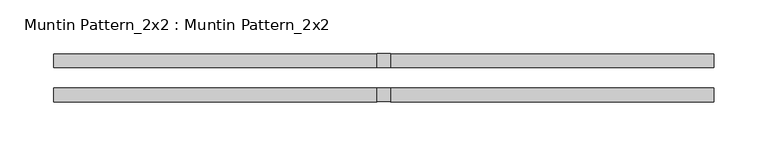
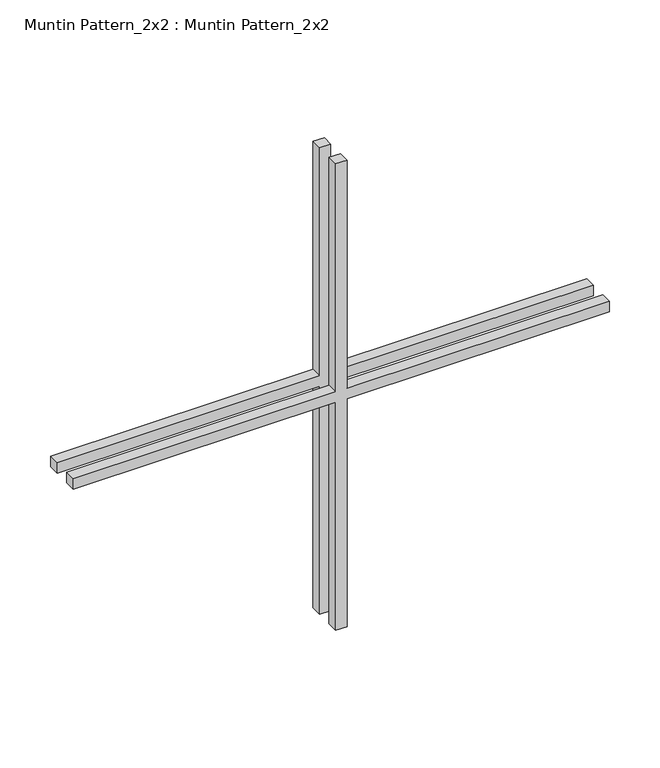
"""IFC4 building model written with IfcOpenShell, lengths in millimetres: proxy geometry, Muntin Pattern_2x2 : Muntin Pattern_2x2."""

from ifc_helpers import new_model, si_unit, frame, origin, place, context, project, spatial, polyline, outline, extrude, source, transform, mapped, element, save


def muntin_pattern_2x2_muntin_pattern_2x2_bf2d4cb0(model_context):
    return source(origin(), model_context, "Body", "SweptSolid", [
        extrude(outline(polyline([(287.3375, -6.35), (287.3375, -305.59375), (274.6375, -305.59375), (274.6375, -6.35), (0.0, -6.35), (0.0, 6.35), (274.6375, 6.35), (274.6375, 305.59375), (287.3375, 305.59375), (287.3375, 6.35), (561.975, 6.35), (561.975, -6.35), (287.3375, -6.35)])), frame((0.0, 9.525, 0.0), z_axis=(0.0, 1.0, 0.0), x_axis=(0.0, 0.0, 1.0)), (0.0, 0.0, 1.0), 12.7),
        extrude(outline(polyline([(287.3375, -6.35), (287.3375, -305.59375), (274.6375, -305.59375), (274.6375, -6.35), (0.0, -6.35), (0.0, 6.35), (274.6375, 6.35), (274.6375, 305.59375), (287.3375, 305.59375), (287.3375, 6.35), (561.975, 6.35), (561.975, -6.35), (287.3375, -6.35)])), frame((0.0, -22.225, 0.0), z_axis=(0.0, 1.0, 0.0), x_axis=(0.0, 0.0, 1.0)), (0.0, 0.0, 1.0), 12.7),
    ])


if __name__ == "__main__":
    model = new_model("IFC4")
    model_context = context("Model", 3, world=origin())
    ifc_project = project(units=[si_unit("LENGTHUNIT", "METRE", prefix="MILLI")], contexts=[model_context])
    site = spatial("IfcSite", under=ifc_project)
    building = spatial("IfcBuilding", under=site)
    placement = place(None, origin())
    muntin_pattern_2x2_muntin_pattern_2x2_shape = muntin_pattern_2x2_muntin_pattern_2x2_bf2d4cb0(model_context)
    element("IfcBuildingElementProxy", 1, Name="Muntin Pattern_2x2 : Muntin Pattern_2x2", ObjectType="Muntin Pattern_2x2 : Muntin Pattern_2x2", at=placement, inside=building, context=model_context, shape_type="MappedRepresentation", body=[
        mapped(muntin_pattern_2x2_muntin_pattern_2x2_shape, transform((0.0, 0.0, 0.0), x_axis=(1.0, 0.0, 0.0), y_axis=(0.0, 1.0, 0.0), z_axis=(0.0, 0.0, 1.0))),
    ])
    save(model, "model.ifc")

# Revit data of these elements
# Type "Muntin Pattern_2x2 : Muntin Pattern_2x2"
#   Width [instance default] = 4' - 0"
#   Thickness = 0' - 0 1/2"
#   Height [instance default] = 4' - 0"
#   Distance = 0' - 0 3/4"
#   Interior Material [instance default] = none
#   Exterior Material [instance default] = none
#   Default Elevation = 0
# Element 1 (IfcBuildingElementProxy, "Muntin Pattern_2x2 : Muntin Pattern_2x2")
#   Width = 2' - 0 1/16"
#   Height = 1' - 10 1/8"
#   Interior Material = Wood - Stained
#   Exterior Material = Clad - White
#   Materials on its faces: "Clad - White", "Wood - Stained"
# Materials
#   "Clad - White": class "Wood", colour RGB 242 242 238, transparency 0, Cost = 0
#   "Wood - Stained": class "Wood", colour RGB 224 178 126, transparency 0, Cost = 0
